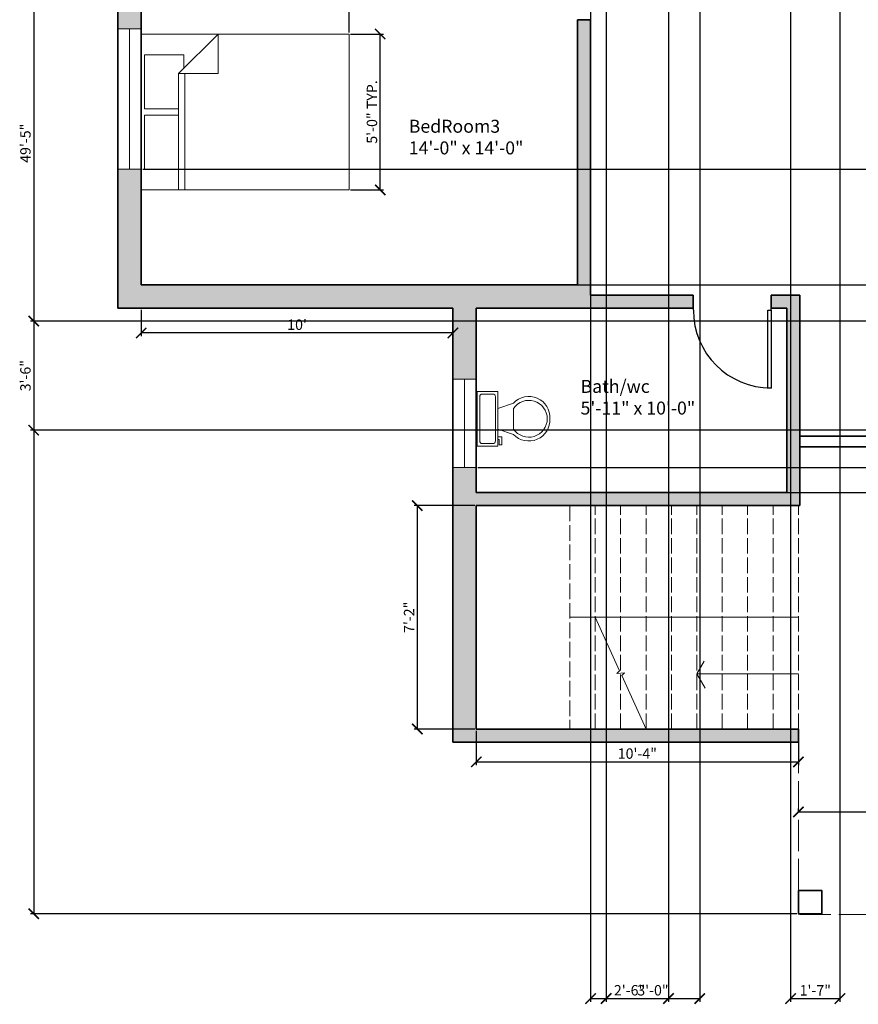
# Model space of a CAD drawing. Units: inches. Extents: x -43 to 8979, y -615 to 8149.
# Tile 1 of 5: x -40 to 283, y -614 to -235. Entities that reach past the tile are written whole.
import ezdxf

# ---------------------------------------------------------------- set-up
doc = ezdxf.new("R2010")
doc.units = ezdxf.units.IN
doc.header["$PDMODE"] = 35
doc.header["$PDSIZE"] = 5
doc.linetypes.add('ACAD_ISO02W100', pattern=[15, 12, -3])
for name, color, linetype, lineweight in [('A-ANNO-DIMS', 2, 'Continuous', 18), ('A-AREA-IDEN', 7, 'Continuous', 25), ('A-COLS', 7, 'Continuous', 35), ('A-DOOR', 4, 'Continuous', 25), ('A-FLOR-FIXT', 9, 'Continuous', 18), ('A-FLOR-PRKG', 8, 'ACAD_ISO02W100', 18), ('A-FLOR-STRS', 3, 'Continuous', 18), ('A-FLOR-STRS-OVHD', 3, 'ACAD_ISO02W100', 18), ('A-FURN', 9, 'Continuous', 18), ('A-GLAZ', 4, 'Continuous', 18), ('A-WALL', 7, 'Continuous', 35), ('A-WALL-PATT', 1, 'Continuous', 13)]:
    doc.layers.add(name, color=color, linetype=linetype, lineweight=lineweight)
doc.styles.get("Standard").update_dxf_attribs({"font": 'arial.ttf'})
doc.dimstyles.new('ISO-25', dxfattribs={"dimtxt": 4, "dimasz": 4, "dimexe": 1.25, "dimexo": 0.625, "dimtad": 1, "dimlunit": 3, "dimtxsty": 'Standard', "dimblk": 'ARCHTICK', "dimcen": 2.5, "dimadec": 0, "dimazin": 0, "dimtfac": 1, "dimtmove": 0, "dimatfit": 3, "dimfxl": 1, "dimarcsym": 0})

# ---------------------------------------------------------------- blocks, each defined once
blk = doc.blocks.new('*U3')
for p, q in [((0, 0), (0, -6)), ((40, 0), (40, -6))]:
    blk.add_line(p, q)
blk.add_lwpolyline([(0, 0), (0, 40), (1.75, 40), (1.75, 0)], close=True)
blk.add_arc((0, 0), 40, 0, 90)
blk = doc.blocks.new('Bed - Queen')
for p, q in [((0, -80.00003), (0, 0)), ((0, 0), (59.99999, 0)), ((59.99999, 0), (59.99999, -80.00003)), ((7.99999, -1.2), (28.79998, -1.2)), ((7.99999, -14.4), (7.99999, -1.2)), ((28.79998, -1.2), (28.79998, -14.4)), ((31.19999, -1.2), (51.99999, -1.2)), ((31.19999, -14.4), (31.19999, -1.2)), ((51.99999, -1.2), (51.99999, -16.4)), ((0, -14.4), (44.8, -14.4)), ((59.99999, -29.6), (44.8, -14.4)), ((44.8, -14.4), (44.8, -29.6)), ((44.8, -16.8), (0, -16.8)), ((51.99999, -16.4), (46.79936, -16.4)), ((44.8, -29.6), (59.99999, -29.6)), ((59.99999, -80.00003), (0, -80.00003))]:
    blk.add_line(p, q)
blk = doc.blocks.new('*U7')
for p, q in [((9.5, -6), (9.5, -2)), ((-10, -8.5), (-8, -8.5)), ((-10, -9.5), (-10, -8.5)), ((-7, -9.5), (-10, -9.5)), ((-8, -8.5), (-8, -8)), ((-7, -8), (-7, -9.5)), ((-4, -8), (-6, -14)), ((4, -8), (6, -14)), ((4, -14), (-4, -14))]:
    blk.add_line(p, q)
blk.add_lwpolyline([(10.5, -8), (10.5, 0), (-10.5, 0), (-10.5, -8)], close=True)
for points in [[(-9.5, -2), (-9.5, -6)], [(8.5, -1), (-8.5, -1)], [(-8.5, -7), (8.5, -7)]]:
    blk.add_lwpolyline(points)
for centre, radius, start, end in [((-8.625, -1.875), 0.8839, 81.8699, 188.1301), ((8.625, -1.875), 0.8839, 351.8699, 98.1301), ((-8.625, -6.125), 0.8839, 171.869898, 278.1301), ((8.625, -6.125), 0.8839, 261.8699, 8.1301), ((-0.4772, -19.9188), 8.0953, 133.01722, 273.38), ((0.0374, -19.8731), 7.127, 124.50543, 269.7), ((-0.0373, -19.8731), 7.127, 270.3, 55.4946), ((0.4773, -19.9188), 8.0953, 266.62, 46.9828)]:
    blk.add_arc(centre, radius, start, end)
blk = doc.blocks.new('_ArchTick')
at = {"color": 0, "linetype": 'ByBlock', "const_width": 0.15}
blk.add_lwpolyline([(-0.5, -0.5), (0.5, 0.5)], dxfattribs=at)
blk = doc.blocks.new('*D14')
at = {"layer": 'A-ANNO-DIMS', "color": 0, "lineweight": -2, "transparency": 16777216}
for p, q in [((260.05, -539.77), (260.05, -538.32)), ((260.05, -539.57), (389.05, -539.57)), ((389.05, -545.24), (389.05, -538.32))]:
    blk.add_line(p, q, dxfattribs=at)
at = {"layer": 'Defpoints', "color": 0, "transparency": 16777216}
for p in [(260.05, -540.39), (389.05, -539.57), (389.05, -545.87)]:
    blk.add_point(p, dxfattribs=at)
at = {"layer": 'A-ANNO-DIMS', "color": 0, "lineweight": -2, "transparency": 16777216, "xscale": 4, "yscale": 4, "zscale": 4, "rotation": 180}
blk.add_blockref('_ArchTick', (260.05, -539.57), dxfattribs=at)
at = {"layer": 'A-ANNO-DIMS', "color": 0, "lineweight": -2, "transparency": 16777216, "xscale": 4, "yscale": 4, "zscale": 4}
blk.add_blockref('_ArchTick', (389.05, -539.57), dxfattribs=at)
at = {"layer": 'A-ANNO-DIMS', "color": 0, "transparency": 16777216, "insert": (324.55, -536.9), "char_height": 4, "attachment_point": 5}
blk.add_mtext('11\'-6"', dxfattribs=at)
blk = doc.blocks.new('*D15')
at = {"layer": 'A-ANNO-DIMS', "color": 0, "lineweight": -2, "transparency": 16777216}
for p, q in [((135.43, -421.7), (112.07, -421.7)), ((113.32, -421.7), (113.32, -507.7)), ((135.43, -507.7), (112.07, -507.7))]:
    blk.add_line(p, q, dxfattribs=at)
at = {"layer": 'Defpoints', "color": 0, "transparency": 16777216}
for p in [(136.05, -421.7), (113.32, -507.7), (136.05, -507.7)]:
    blk.add_point(p, dxfattribs=at)
at = {"layer": 'A-ANNO-DIMS', "color": 0, "lineweight": -2, "transparency": 16777216, "xscale": 4, "yscale": 4, "zscale": 4}
for p, rotation in [((113.32, -421.7), 90), ((113.32, -507.7), 270)]:
    blk.add_blockref('_ArchTick', p, dxfattribs=dict(at, rotation=rotation))
at = {"layer": 'A-ANNO-DIMS', "color": 0, "transparency": 16777216, "insert": (110.69, -464.7), "char_height": 4, "attachment_point": 5, "rotation": 90}
blk.add_mtext('7\'-2"', dxfattribs=at)
blk = doc.blocks.new('*D16')
at = {"layer": 'A-ANNO-DIMS', "color": 0, "lineweight": -2, "transparency": 16777216}
for p, q in [((136.05, -508.33), (136.05, -521.58)), ((260.05, -508.33), (260.05, -521.58)), ((136.05, -520.33), (260.05, -520.33))]:
    blk.add_line(p, q, dxfattribs=at)
at = {"layer": 'Defpoints', "color": 0, "transparency": 16777216}
for p in [(136.05, -507.7), (260.05, -507.7), (260.05, -520.33)]:
    blk.add_point(p, dxfattribs=at)
at = {"layer": 'A-ANNO-DIMS', "color": 0, "lineweight": -2, "transparency": 16777216, "xscale": 4, "yscale": 4, "zscale": 4, "rotation": 180}
blk.add_blockref('_ArchTick', (136.05, -520.33), dxfattribs=at)
at = {"layer": 'A-ANNO-DIMS', "color": 0, "lineweight": -2, "transparency": 16777216, "xscale": 4, "yscale": 4, "zscale": 4}
blk.add_blockref('_ArchTick', (260.05, -520.33), dxfattribs=at)
at = {"layer": 'A-ANNO-DIMS', "color": 0, "transparency": 16777216, "insert": (198.05, -517.66), "char_height": 4, "attachment_point": 5}
blk.add_mtext('10\'-4"', dxfattribs=at)
blk = doc.blocks.new('*D17')
at = {"layer": 'A-ANNO-DIMS', "color": 0, "lineweight": -2, "transparency": 16777216}
for p, q in [((7.05, -346.33), (7.05, -356.51)), ((127.05, -346.33), (127.05, -356.51)), ((127.05, -355.26), (7.05, -355.26))]:
    blk.add_line(p, q, dxfattribs=at)
at = {"layer": 'Defpoints', "color": 0, "transparency": 16777216}
for p in [(7.05, -345.7), (127.05, -345.7), (7.05, -355.26)]:
    blk.add_point(p, dxfattribs=at)
at = {"layer": 'A-ANNO-DIMS', "color": 0, "lineweight": -2, "transparency": 16777216, "xscale": 4, "yscale": 4, "zscale": 4, "rotation": 180}
blk.add_blockref('_ArchTick', (7.05, -355.26), dxfattribs=at)
at = {"layer": 'A-ANNO-DIMS', "color": 0, "lineweight": -2, "transparency": 16777216, "xscale": 4, "yscale": 4, "zscale": 4}
blk.add_blockref('_ArchTick', (127.05, -355.26), dxfattribs=at)
at = {"layer": 'A-ANNO-DIMS', "color": 0, "transparency": 16777216, "insert": (67.05, -352.59), "char_height": 4, "attachment_point": 5}
blk.add_mtext("10'", dxfattribs=at)
blk = doc.blocks.new('WIN-54x9')
blk.add_line((4.5, 0), (4.5, 54))
blk.add_lwpolyline([(0, 0), (0, 54), (9, 54), (9, 0)], close=True)
blk = doc.blocks.new('WIN-34x9')
blk.add_line((4.5, 0), (4.5, 34))
blk.add_lwpolyline([(0, 0), (0, 34), (9, 34), (9, 0)], close=True)
blk = doc.blocks.new('POST-9x9')
blk.add_lwpolyline([(0, 9), (9, 9), (9, 0), (0, 0)], close=True)
blk = doc.blocks.new('*D23')
at = {"layer": 'A-ANNO-DIMS', "color": 0, "lineweight": -2, "transparency": 16777216}
for p, q in [((7.05, -239.58), (7.05, -226.96)), ((87.05, -239.58), (87.05, -226.96)), ((87.05, -228.21), (7.05, -228.21))]:
    blk.add_line(p, q, dxfattribs=at)
at = {"layer": 'Defpoints', "color": 0, "transparency": 16777216}
for p in [(7.05, -228.21), (7.05, -240.21), (87.05, -240.21)]:
    blk.add_point(p, dxfattribs=at)
at = {"layer": 'A-ANNO-DIMS', "color": 0, "lineweight": -2, "transparency": 16777216, "xscale": 4, "yscale": 4, "zscale": 4, "rotation": 180}
blk.add_blockref('_ArchTick', (7.05, -228.21), dxfattribs=at)
at = {"layer": 'A-ANNO-DIMS', "color": 0, "lineweight": -2, "transparency": 16777216, "xscale": 4, "yscale": 4, "zscale": 4}
blk.add_blockref('_ArchTick', (87.05, -228.21), dxfattribs=at)
at = {"layer": 'A-ANNO-DIMS', "color": 0, "transparency": 16777216, "insert": (47.05, -225.39), "char_height": 4, "attachment_point": 5}
blk.add_mtext('QUEEN BED 6\'-8" TYP.', dxfattribs=at)
blk = doc.blocks.new('*D24')
at = {"layer": 'A-ANNO-DIMS', "color": 0, "lineweight": -2, "transparency": 16777216}
for p, q in [((87.68, -240.21), (100.3, -240.21)), ((99.05, -300.21), (99.05, -240.21)), ((87.68, -300.21), (100.3, -300.21))]:
    blk.add_line(p, q, dxfattribs=at)
at = {"layer": 'Defpoints', "color": 0, "transparency": 16777216}
for p in [(87.05, -240.21), (99.05, -240.21), (87.05, -300.21)]:
    blk.add_point(p, dxfattribs=at)
at = {"layer": 'A-ANNO-DIMS', "color": 0, "lineweight": -2, "transparency": 16777216, "xscale": 4, "yscale": 4, "zscale": 4}
for p, rotation in [((99.05, -240.21), 90), ((99.05, -300.21), 270)]:
    blk.add_blockref('_ArchTick', p, dxfattribs=dict(at, rotation=rotation))
at = {"layer": 'A-ANNO-DIMS', "color": 0, "transparency": 16777216, "insert": (96.39, -270.21), "char_height": 4, "attachment_point": 5, "rotation": 90}
blk.add_mtext('5\'-0" TYP.', dxfattribs=at)
blk = doc.blocks.new('*D43')
at = {"layer": 'A-ANNO-DIMS', "color": 0, "lineweight": -2, "transparency": 16777216}
for p, q in [((257.05, 4.67), (257.05, -612.69)), ((276.05, 4.67), (276.05, -612.69)), ((257.05, -611.44), (276.05, -611.44))]:
    blk.add_line(p, q, dxfattribs=at)
at = {"layer": 'Defpoints', "color": 0, "transparency": 16777216}
for p in [(257.05, 5.3), (276.05, 5.3), (276.05, -611.44)]:
    blk.add_point(p, dxfattribs=at)
at = {"layer": 'A-ANNO-DIMS', "color": 0, "lineweight": -2, "transparency": 16777216, "xscale": 4, "yscale": 4, "zscale": 4, "rotation": 180}
blk.add_blockref('_ArchTick', (257.05, -611.44), dxfattribs=at)
at = {"layer": 'A-ANNO-DIMS', "color": 0, "lineweight": -2, "transparency": 16777216, "xscale": 4, "yscale": 4, "zscale": 4}
blk.add_blockref('_ArchTick', (276.05, -611.44), dxfattribs=at)
at = {"layer": 'A-ANNO-DIMS', "color": 0, "transparency": 16777216, "insert": (266.55, -608.8), "char_height": 4, "attachment_point": 5}
blk.add_mtext('1\'-7"', dxfattribs=at)
blk = doc.blocks.new('*D46')
at = {"layer": 'A-ANNO-DIMS', "color": 0, "lineweight": -2, "transparency": 16777216}
for p, q in [((7.68, -292.21), (552.7, -292.21)), ((551.45, -336.7), (551.45, -292.21)), ((7.68, -336.7), (552.7, -336.7))]:
    blk.add_line(p, q, dxfattribs=at)
at = {"layer": 'Defpoints', "color": 0, "transparency": 16777216}
for p in [(7.05, -292.21), (551.45, -292.21), (7.05, -336.7)]:
    blk.add_point(p, dxfattribs=at)
at = {"layer": 'A-ANNO-DIMS', "color": 0, "lineweight": -2, "transparency": 16777216, "xscale": 4, "yscale": 4, "zscale": 4}
for p, rotation in [((551.45, -292.21), 90), ((551.45, -336.7), 270)]:
    blk.add_blockref('_ArchTick', p, dxfattribs=dict(at, rotation=rotation))
at = {"layer": 'A-ANNO-DIMS', "color": 0, "transparency": 16777216, "insert": (548.76, -314.45), "char_height": 4, "attachment_point": 5, "rotation": 90}
blk.add_mtext('3\'-8 1/2"', dxfattribs=at)
blk = doc.blocks.new('*D47')
at = {"layer": 'A-ANNO-DIMS', "color": 0, "lineweight": -2, "transparency": 16777216}
for p, q in [((551.45, -407.03), (551.45, -381.83)), ((136.68, -407.03), (552.7, -407.03)), ((551.45, -416.7), (551.45, -407.03)), ((136.68, -416.7), (552.7, -416.7))]:
    blk.add_line(p, q, dxfattribs=at)
at = {"layer": 'Defpoints', "color": 0, "transparency": 16777216}
for p in [(136.05, -407.03), (551.45, -407.03), (136.05, -416.7)]:
    blk.add_point(p, dxfattribs=at)
at = {"layer": 'A-ANNO-DIMS', "color": 0, "lineweight": -2, "transparency": 16777216, "xscale": 4, "yscale": 4, "zscale": 4}
for p, rotation in [((551.45, -407.03), 90), ((551.45, -416.7), 270)]:
    blk.add_blockref('_ArchTick', p, dxfattribs=dict(at, rotation=rotation))
at = {"layer": 'A-ANNO-DIMS', "color": 0, "transparency": 16777216, "insert": (548.76, -392.43), "char_height": 4, "attachment_point": 5, "rotation": 90}
blk.add_mtext('0\'-9 1/2"', dxfattribs=at)
blk = doc.blocks.new('*D53')
at = {"layer": 'A-ANNO-DIMS', "color": 0, "lineweight": -2, "transparency": 16777216}
for p, q in [((-2.57, 14.3), (-35.6, 14.3)), ((-34.35, 14.3), (-34.35, -578.78)), ((259.43, -578.78), (-35.6, -578.78))]:
    blk.add_line(p, q, dxfattribs=at)
at = {"layer": 'Defpoints', "color": 0, "transparency": 16777216}
for p in [(-1.95, 14.3), (-34.35, -578.78), (260.05, -578.78)]:
    blk.add_point(p, dxfattribs=at)
at = {"layer": 'A-ANNO-DIMS', "color": 0, "lineweight": -2, "transparency": 16777216, "xscale": 4, "yscale": 4, "zscale": 4}
for p, rotation in [((-34.35, 14.3), 90), ((-34.35, -578.78), 270)]:
    blk.add_blockref('_ArchTick', p, dxfattribs=dict(at, rotation=rotation))
at = {"layer": 'A-ANNO-DIMS', "color": 0, "transparency": 16777216, "insert": (-37.01, -282.24), "char_height": 4, "attachment_point": 5, "rotation": 90}
blk.add_mtext('49\'-5"', dxfattribs=at)
blk = doc.blocks.new('*D54')
at = {"layer": 'A-ANNO-DIMS', "color": 0, "lineweight": -2, "transparency": 16777216}
for p, q in [((180.05, -108.33), (180.05, -612.69)), ((210.05, -108.33), (210.05, -612.69)), ((180.05, -611.44), (210.05, -611.44))]:
    blk.add_line(p, q, dxfattribs=at)
at = {"layer": 'Defpoints', "color": 0, "transparency": 16777216}
for p in [(180.05, -107.7), (210.05, -107.7), (210.05, -611.44)]:
    blk.add_point(p, dxfattribs=at)
at = {"layer": 'A-ANNO-DIMS', "color": 0, "lineweight": -2, "transparency": 16777216, "xscale": 4, "yscale": 4, "zscale": 4, "rotation": 180}
blk.add_blockref('_ArchTick', (180.05, -611.44), dxfattribs=at)
at = {"layer": 'A-ANNO-DIMS', "color": 0, "lineweight": -2, "transparency": 16777216, "xscale": 4, "yscale": 4, "zscale": 4}
blk.add_blockref('_ArchTick', (210.05, -611.44), dxfattribs=at)
at = {"layer": 'A-ANNO-DIMS', "color": 0, "transparency": 16777216, "insert": (195.05, -608.77), "char_height": 4, "attachment_point": 5}
blk.add_mtext('2\'-6"', dxfattribs=at)
blk = doc.blocks.new('*D55')
at = {"layer": 'A-ANNO-DIMS', "color": 0, "lineweight": -2, "transparency": 16777216}
for p, q in [((186.05, -169.33), (186.05, -612.69)), ((222.05, -169.33), (222.05, -612.69)), ((186.05, -611.44), (222.05, -611.44))]:
    blk.add_line(p, q, dxfattribs=at)
at = {"layer": 'Defpoints', "color": 0, "transparency": 16777216}
for p in [(186.05, -168.7), (222.05, -168.7), (222.05, -611.44)]:
    blk.add_point(p, dxfattribs=at)
at = {"layer": 'A-ANNO-DIMS', "color": 0, "lineweight": -2, "transparency": 16777216, "xscale": 4, "yscale": 4, "zscale": 4, "rotation": 180}
blk.add_blockref('_ArchTick', (186.05, -611.44), dxfattribs=at)
at = {"layer": 'A-ANNO-DIMS', "color": 0, "lineweight": -2, "transparency": 16777216, "xscale": 4, "yscale": 4, "zscale": 4}
blk.add_blockref('_ArchTick', (222.05, -611.44), dxfattribs=at)
at = {"layer": 'A-ANNO-DIMS', "color": 0, "transparency": 16777216, "insert": (204.05, -608.77), "char_height": 4, "attachment_point": 5}
blk.add_mtext('3\'-0"', dxfattribs=at)
blk = doc.blocks.new('*D56')
at = {"layer": 'A-ANNO-DIMS', "color": 0, "lineweight": -2, "transparency": 16777216}
for p, q in [((388.43, -350.7), (-35.6, -350.7)), ((-34.35, -350.7), (-34.35, -392.7)), ((388.43, -392.7), (-35.6, -392.7))]:
    blk.add_line(p, q, dxfattribs=at)
at = {"layer": 'Defpoints', "color": 0, "transparency": 16777216}
for p in [(389.05, -350.7), (-34.35, -392.7), (389.05, -392.7)]:
    blk.add_point(p, dxfattribs=at)
at = {"layer": 'A-ANNO-DIMS', "color": 0, "lineweight": -2, "transparency": 16777216, "xscale": 4, "yscale": 4, "zscale": 4}
for p, rotation in [((-34.35, -350.7), 90), ((-34.35, -392.7), 270)]:
    blk.add_blockref('_ArchTick', p, dxfattribs=dict(at, rotation=rotation))
at = {"layer": 'A-ANNO-DIMS', "color": 0, "transparency": 16777216, "insert": (-37.01, -371.7), "char_height": 4, "attachment_point": 5, "rotation": 90}
blk.add_mtext('3\'-6"', dxfattribs=at)

msp = doc.modelspace()

# ---------------------------------------------------------------- hatches: boundary and pattern name
at = {"layer": 'A-WALL-PATT'}
h = msp.add_hatch(color=256, dxfattribs=at)
h.dxf.hatch_style = 1
h.paths.add_polyline_path([(7.054, 5.297), (58.783, 5.297), (58.783, 14.297), (-1.946, 14.297), (-1.946, -51.444), (7.054, -51.444)])
h.paths.add_polyline_path([(7.054, -105.444), (-1.946, -105.444), (-1.946, -238.206), (7.054, -238.206), (7.054, -168.703), (175.054, -168.703), (180.054, -168.703), (186.046, -168.703), (186.046, -163.703), (175.054, -163.703), (7.054, -163.703)])
h.paths.add_polyline_path([(199.054, 14.297), (112.783, 14.297), (112.783, 5.297), (116.889, 5.297), (175.054, 5.297), (175.054, -107.703), (180.054, -107.703), (180.054, -103.21), (180.054, -73.263), (180.054, 5.297), (199.054, 5.297)])
h.paths.add_polyline_path([(276.054, 14.297), (233.054, 14.297), (233.054, 5.297), (252.054, 5.297), (252.054, -102.703), (210.054, -102.703), (210.054, -107.703), (252.054, -107.703), (252.054, -163.703), (222.054, -163.703), (222.054, -168.703), (286.948, -168.703), (286.948, -163.703), (257.054, -163.703), (257.054, -107.703), (299.054, -107.703), (299.054, -102.703), (257.054, -102.703), (257.054, 5.297), (276.054, 5.297)])
h.paths.add_polyline_path([(417.209, 14.297), (310.054, 14.297), (310.054, 5.297), (329.054, 5.297), (329.054, -107.703), (334.054, -107.703), (334.054, 5.297), (417.209, 5.297)])
h.paths.add_polyline_path([(519.054, 14.297), (471.209, 14.297), (471.209, 5.297), (514.054, 5.297), (514.054, -20.367), (519.054, -20.367)])
h.paths.add_polyline_path([(519.054, -74.367), (514.054, -74.367), (514.054, -163.703), (323.054, -163.703), (323.054, -168.703), (329.054, -168.703), (334.054, -168.703), (389.054, -168.703), (389.054, -210.703), (394.054, -210.703), (394.054, -168.703), (514.054, -168.703), (514.054, -194.4), (519.054, -194.4)])
h.paths.add_polyline_path([(519.054, -248.4), (514.054, -248.4), (514.054, -252.703), (394.054, -252.703), (394.054, -246.703), (389.054, -246.703), (389.054, -263.703), (394.054, -263.703), (394.054, -257.703), (514.054, -257.703), (514.054, -264.224), (519.054, -264.224)])
h = msp.add_hatch(color=256, dxfattribs=at)
h.dxf.hatch_style = 1
h.paths.add_polyline_path([(519.054, -318.224), (514.054, -318.224), (514.054, -341.703), (394.054, -341.703), (394.054, -299.703), (389.054, -299.703), (389.054, -341.703), (389.054, -346.703), (389.054, -350.703), (394.054, -350.703), (394.054, -346.703), (514.054, -346.703), (514.054, -424.484), (519.054, -424.484)])
h.paths.add_polyline_path([(519.054, -478.484), (514.054, -478.484), (514.054, -479.58), (514.054, -507.703), (394.054, -507.703), (394.054, -392.703), (389.054, -392.703), (389.054, -512.703), (394.054, -512.703), (519.054, -512.703)])
h.paths.add_polyline_path([(136.054, -421.703), (260.554, -421.703), (260.554, -416.703), (260.554, -345.703), (260.554, -340.703), (249.554, -340.703), (249.554, -345.703), (255.554, -345.703), (255.554, -416.703), (136.054, -416.703), (136.054, -407.032), (127.054, -407.032), (127.054, -512.703), (260.054, -512.703), (260.054, -507.703), (136.054, -507.703)])
h.paths.add_polyline_path([(219.554, -340.703), (180.054, -340.703), (180.054, -234.703), (175.054, -234.703), (175.054, -336.703), (7.054, -336.703), (7.054, -292.206), (-1.946, -292.206), (-1.946, -345.703), (127.054, -345.703), (127.054, -373.032), (136.054, -373.032), (136.054, -345.703), (180.054, -345.703), (219.554, -345.703)])

# ---------------------------------------------------------------- linework, layer by layer
at = {"layer": 'A-FLOR-PRKG'}
for p, q in [((260.054, -512.703), (260.054, -579.037)), ((260.554, -579.037), (389.054, -579.037))]:
    msp.add_line(p, q, dxfattribs=at)
at = {"layer": 'A-FLOR-STRS'}
for p, q in [((172.054, -464.703), (260.054, -464.703)), ((220.943, -486.474), (223.732, -481.644)), ((220.943, -486.474), (260.054, -486.474)), ((220.943, -486.474), (224.132, -491.997))]:
    msp.add_line(p, q, dxfattribs=at)
msp.add_lwpolyline([(181.832, -464.703), (191.196, -485.292), (190.153, -486.316), (193.067, -486.089), (192.024, -487.113), (201.388, -507.703)], dxfattribs=at)
at = {"layer": 'A-FLOR-STRS-OVHD', "ltscale": 0.5}
for p, q in [((172.054, -421.703), (172.054, -507.703)), ((181.832, -507.703), (181.832, -421.703)), ((191.61, -507.703), (191.61, -421.703)), ((201.388, -507.703), (201.388, -421.703)), ((211.166, -507.703), (211.166, -421.703)), ((220.943, -507.703), (220.943, -421.703)), ((230.721, -507.703), (230.721, -421.703)), ((240.499, -507.703), (240.499, -421.703)), ((250.277, -507.703), (250.277, -421.703)), ((260.054, -507.703), (260.054, -421.703))]:
    msp.add_line(p, q, dxfattribs=at)
at = {"layer": 'A-WALL'}
for p, q in [((-1.946, -345.703), (-1.946, 14.297)), ((7.054, -336.703), (7.054, -168.703)), ((175.054, -336.703), (175.054, -234.703)), ((175.054, -234.703), (180.054, -234.703)), ((180.054, -340.703), (180.054, -234.703)), ((7.054, -336.703), (175.054, -336.703)), ((180.054, -340.703), (219.554, -340.703)), ((219.554, -345.703), (219.554, -340.703)), ((249.554, -345.703), (249.554, -340.703)), ((249.554, -340.703), (260.554, -340.703)), ((260.554, -345.703), (260.554, -340.703)), ((-1.946, -345.703), (127.054, -345.703)), ((127.054, -345.703), (127.054, -512.703)), ((136.054, -345.703), (136.054, -416.703)), ((136.054, -345.703), (180.054, -345.703)), ((180.054, -345.703), (219.554, -345.703)), ((249.554, -345.703), (255.554, -345.703)), ((255.554, -416.703), (255.554, -345.703)), ((260.554, -416.703), (260.554, -345.703)), ((296.354, -395.037), (260.554, -395.037)), ((295.483, -399.037), (260.554, -399.037)), ((136.054, -416.703), (255.554, -416.703)), ((260.554, -421.703), (260.554, -416.703)), ((136.054, -421.703), (260.554, -421.703)), ((136.054, -421.703), (136.054, -507.703)), ((251.054, -421.703), (256.054, -421.703)), ((136.054, -507.703), (260.054, -507.703)), ((260.054, -507.703), (260.054, -512.703)), ((260.054, -512.703), (127.054, -512.703))]:
    msp.add_line(p, q, dxfattribs=at)

# ---------------------------------------------------------------- block references
at = {"layer": 'A-COLS'}
msp.add_blockref('POST-9x9', (260.054, -578.784), dxfattribs=at)
at = {"layer": 'A-DOOR', "xscale": 0.7486801686032757, "yscale": 0.7486801686032757, "zscale": 0.7486801686032757, "rotation": 180}
msp.add_blockref('*U3', (249.554, -346.498), dxfattribs=at)
at = {"layer": 'A-FLOR-FIXT', "rotation": 90}
msp.add_blockref('*U7', (136.376, -388.28), dxfattribs=at)
at = {"layer": 'A-FURN', "rotation": 90}
msp.add_blockref('Bed - Queen', (7.054, -300.206), dxfattribs=at)
at = {"layer": 'A-GLAZ'}
for name, p in [('WIN-54x9', (-1.946, -292.206)), ('WIN-34x9', (127.054, -407.032))]:
    msp.add_blockref(name, p, dxfattribs=at)

# ---------------------------------------------------------------- texts
at = {"layer": 'A-AREA-IDEN', "char_height": 5, "attachment_point": 1}
for s, width, insert in [('BedRoom3\\P14\'-0" x 14\'-0"', 101.99671, (110.043, -273.197)), ('Bath/wc\\P5\'-11" x 10\'-0"', 52.09042, (176.182, -373.324))]:
    msp.add_mtext_dynamic_manual_height_columns(s, width=width, gutter_width=12.5, heights=[0], dxfattribs=dict(at, insert=insert))

# ---------------------------------------------------------------- dimensions: what is measured, and where the dimension line sits
at = {"layer": 'A-ANNO-DIMS'}
for base, p1, p2, override, picture, middle in [((-34.346, -578.784), (-1.946, 14.297), (260.054, -578.784), {"dimdec": 1, "dimlfac": 1, "dimrnd": 0, "dimzin": 1, "dimdsep": 46, "dimlunit": 4, "dimfrac": 2}, '*D53', (-37.013, -282.243)), ((551.454, -292.206), (7.054, -336.703), (7.054, -292.206), {"dimdec": 1, "dimlfac": 1, "dimrnd": 0, "dimzin": 1, "dimdsep": 46, "dimlunit": 4, "dimfrac": 2}, '*D46', (548.76, -314.454)), ((-34.346, -392.703), (389.054, -350.703), (389.054, -392.703), {"dimdec": 1, "dimlfac": 1, "dimrnd": 0, "dimzin": 1, "dimdsep": 46, "dimlunit": 4, "dimfrac": 2}, '*D56', (-37.014, -371.703)), ((551.454, -407.032), (136.054, -416.703), (136.054, -407.032), {"dimdec": 1, "dimlfac": 1, "dimrnd": 0, "dimzin": 1, "dimdsep": 46, "dimlunit": 4, "dimfrac": 2}, '*D47', (548.761, -392.43)), ((113.319, -507.703), (136.054, -421.703), (136.054, -507.703), {"dimclrd": 0, "dimclre": 0, "dimclrt": 0}, '*D15', (110.686, -464.703))]:
    dim = msp.add_linear_dim(base=base, p1=p1, p2=p2, angle=90, dimstyle='ISO-25', override=override, dxfattribs=at)
    dim.commit()
    dim.dimension.update_dxf_attribs({"geometry": picture, "text_midpoint": middle})
for base, p1, p2, override, picture, middle in [((276.054, -611.437), (257.054, 5.297), (276.054, 5.297), {"dimdec": 1, "dimlfac": 1, "dimrnd": 0, "dimzin": 1, "dimdsep": 46, "dimlunit": 4, "dimfrac": 2}, '*D43', (266.554, -608.804)), ((210.054, -611.437), (180.054, -107.703), (210.054, -107.703), {"dimdec": 1, "dimlfac": 1, "dimrnd": 0, "dimzin": 1, "dimdsep": 46, "dimlunit": 4, "dimfrac": 2}, '*D54', (195.054, -608.77)), ((222.054, -611.437), (186.054, -168.703), (222.054, -168.703), {"dimdec": 1, "dimlfac": 1, "dimrnd": 0, "dimzin": 1, "dimdsep": 46, "dimlunit": 4, "dimfrac": 2}, '*D55', (204.054, -608.769)), ((7.054, -355.261), (127.054, -345.703), (7.054, -345.703), {"dimclrd": 0, "dimclre": 0, "dimclrt": 0}, '*D17', (67.054, -352.594)), ((260.054, -520.328), (136.054, -507.703), (260.054, -507.703), {"dimclrd": 0, "dimclre": 0, "dimclrt": 0}, '*D16', (198.054, -517.661))]:
    dim = msp.add_linear_dim(base=base, p1=p1, p2=p2, dimstyle='ISO-25', override=override, dxfattribs=at)
    dim.commit()
    dim.dimension.update_dxf_attribs({"geometry": picture, "text_midpoint": middle})
for base, p1, p2, angle, text, picture, middle in [((7.054, -228.206), (87.054, -240.206), (7.054, -240.206), 180, 'QUEEN BED <> TYP.', '*D23', (47.054, -225.39)), ((99.054, -240.206), (87.054, -300.206), (87.054, -240.206), 90, '<> TYP.', '*D24', (96.387, -270.206))]:
    dim = msp.add_linear_dim(base=base, p1=p1, p2=p2, angle=angle, text=text, dimstyle='ISO-25', override={"dimdec": 1, "dimlfac": 1, "dimrnd": 0, "dimzin": 1, "dimdsep": 46, "dimlunit": 4, "dimfrac": 2}, dxfattribs=at)
    dim.commit()
    dim.dimension.update_dxf_attribs({"geometry": picture, "text_midpoint": middle})
dim = msp.add_linear_dim(base=(389.054, -539.566), p1=(260.054, -540.391), p2=(389.054, -545.87), text='11\'-6"', dimstyle='ISO-25', override={"dimclrd": 0, "dimclre": 0, "dimclrt": 0}, dxfattribs=at)
dim.commit()
dim.dimension.update_dxf_attribs({"geometry": '*D14', "text_midpoint": (324.554, -536.899)})

doc.saveas('drawing.dxf')
